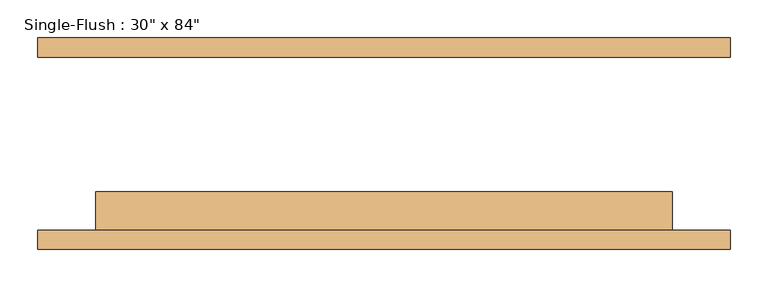
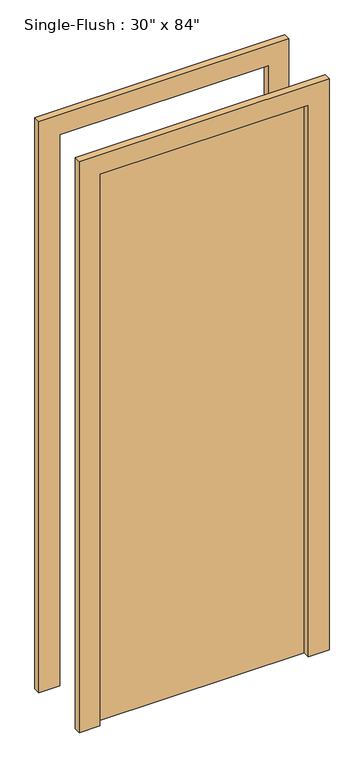
"""IFC4 building model written with IfcOpenShell, lengths in millimetres: door geometry."""

from ifc_helpers import new_model, si_unit, frame, origin, origin_with_axes, place, context, project, spatial, polyline, outline, extrude, source, transform, mapped, element, save


def door_5e1232af(model_context):
    return source(origin(), model_context, "Body", "SweptSolid", [
        extrude(outline(polyline([(2209.8, -457.2), (0.0, -457.2), (0.0, -381.0), (2133.6, -381.0), (2133.6, 381.0), (0.0, 381.0), (0.0, 457.2), (2209.8, 457.2), (2209.8, -457.2)])), frame((0.0, -139.7, 0.0), z_axis=(0.0, 1.0, 0.0), x_axis=(0.0, 0.0, 1.0)), (0.0, 0.0, 1.0), 25.4),
        extrude(outline(polyline([(2209.8, 457.2), (2209.8, -457.2), (0.0, -457.2), (0.0, -381.0), (2133.6, -381.0), (2133.6, 381.0), (0.0, 381.0), (0.0, 457.2), (2209.8, 457.2)])), frame((0.0, 114.3, 0.0), z_axis=(0.0, 1.0, 0.0), x_axis=(0.0, 0.0, 1.0)), (0.0, 0.0, 1.0), 25.4),
        extrude(outline(polyline([(381.0, -63.5), (381.0, -114.3), (-381.0, -114.3), (-381.0, -63.5), (381.0, -63.5)])), origin_with_axes(), (0.0, 0.0, 1.0), 2133.6),
    ])


if __name__ == "__main__":
    model = new_model("IFC4")
    model_context = context("Model", 3, world=origin())
    ifc_project = project(units=[si_unit("LENGTHUNIT", "METRE", prefix="MILLI")], contexts=[model_context])
    site = spatial("IfcSite", under=ifc_project)
    building = spatial("IfcBuilding", under=site)
    placement = place(None, origin())
    door_shape = door_5e1232af(model_context)
    element("IfcDoor", 1, ObjectType="Single-Flush : 30\" x 84\"", at=placement, inside=building, context=model_context, shape_type="MappedRepresentation", body=[
        mapped(door_shape, transform((0.0, 0.0, 0.0), x_axis=(1.0, 0.0, 0.0), y_axis=(0.0, 1.0, 0.0), z_axis=(0.0, 0.0, 1.0))),
    ])
    save(model, "model.ifc")

# Revit data of these elements
# Type "Single-Flush : 30\" x 84\""
#   Type Mark = "4"
#   Construction Type Id = "MDOOR"
#   Assembly Code = "C1020"
#   Analytic Construction = "Metal"
#   Thickness = 0' - 2"
#   Heat Transfer Coefficient (U) = 0.651978 BTU/(h·ft²·°F)
#   Height = 7' - 0"
#   Trim Projection Ext = 0' - 1"
#   Trim Projection Int = 0' - 1"
#   Trim Width = 0' - 3"
#   Width = 2' - 6"
#   Define Thermal Properties by = 1
#   Define Thermal Properties by = 1
#   Door Material = Door - Panel
#   Frame Material = Door - Frame
#   Visual Light Transmittance = 0
#   Solar Heat Gain Coefficient = 0
#   Function = (empty or 0)
#   Wall Closure = (empty or 0)
# Element 1 (IfcDoor, "Single-Flush : 30\" x 84\"")
#   Materials on its faces: "Door - Frame", "Door - Panel"
# Materials
#   "Door - Panel": class "Wood", colour RGB 210 159 95, transparency 0, Cost = 0
#   "Door - Frame": colour RGB 118 70 51, transparency 0, Cost = 0
